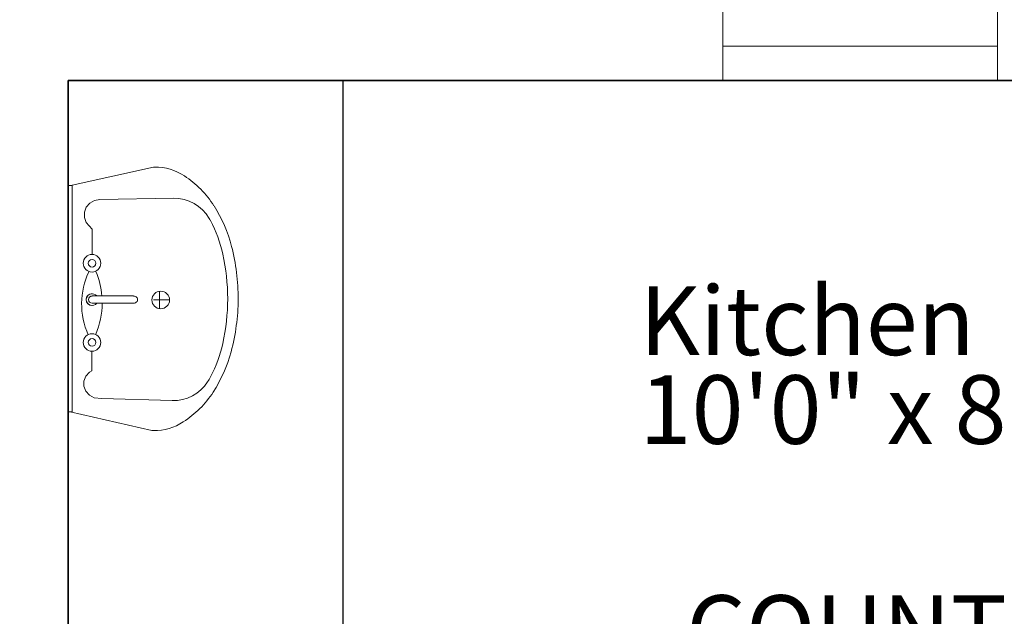
# Model space of a CAD drawing. Units: inches. Extents: x -1198 to -69, y -512 to 437.
# Tile 40 of 50: x -696 to -610, y 210 to 263. Entities that reach past the tile are written whole.
import ezdxf

# ---------------------------------------------------------------- set-up
doc = ezdxf.new("R2010")
doc.units = ezdxf.units.IN
doc.header["$MEASUREMENT"] = 0
for name, color, linetype, lineweight in [('A-ANNO-DIMS', 2, 'Continuous', 18), ('A-AREA-IDEN', 7, 'Continuous', 18), ('A-FLOR-CASE', 7, 'Continuous', 25), ('A-FLOR-FIXT', 60, 'Continuous', 18), ('A-WALL', 7, 'Continuous', 35), ('windows', 160, 'Continuous', 18)]:
    doc.layers.add(name, color=color, linetype=linetype, lineweight=lineweight)
doc.styles.get("Standard").update_dxf_attribs({"font": 'arial.ttf'})
doc.dimstyles.get("Standard").update_dxf_attribs({"dimtxt": 6, "dimasz": 6, "dimexe": 0.18, "dimexo": 0.0625, "dimgap": 0.09, "dimtad": 0, "dimtih": 1, "dimtoh": 1, "dimdec": 0, "dimzin": 0, "dimdsep": 46, "dimlunit": 4, "dimtxsty": 'Standard', "dimblk": 'OBLIQUE', "dimcen": 0.09, "dimadec": 0, "dimazin": 0, "dimtfac": 1, "dimtdec": 0, "dimtofl": 0, "dimtmove": 0, "dimatfit": 3, "dimfxl": 1, "dimtolj": 1, "dimtzin": 0, "dimarcsym": 0})

# ---------------------------------------------------------------- blocks, each defined once
blk = doc.blocks.new('A$C6AA41FE3')
at = {"linetype": 'ByBlock'}
for p, q in [((0.1919, 0.5849), (0.3733, 0.5439)), ((0.3687, 0.04), (0.3687, 0.5439)), ((0.3687, 0.5439), (0.3772, 0.5439)), ((0.3772, 0.0411), (0.3772, 0.5439)), ((0.3026, 0.514), (0.1469, 0.5187)), ((0.32, 0.5127), (0.3026, 0.514)), ((0.3305, 0.5069), (0.32, 0.5127)), ((0.3383, 0.4979), (0.3305, 0.5069)), ((0.3425, 0.4869), (0.3383, 0.4979)), ((0.3425, 0.4752), (0.3425, 0.4869)), ((0.3305, 0.4553), (0.3383, 0.4642)), ((0.3383, 0.4642), (0.3425, 0.4752)), ((0.3251, 0.409), (0.3253, 0.4524)), ((0.3253, 0.4524), (0.3305, 0.4553)), ((0.1747, 0.3146), (0.1747, 0.2774)), ((0.1525, 0.2951), (0.1884, 0.2951)), ((0.2326, 0.3025), (0.3243, 0.3025)), ((0.2326, 0.3021), (0.2326, 0.3025)), ((0.2326, 0.2863), (0.2326, 0.2867)), ((0.3243, 0.2863), (0.2326, 0.2863)), ((0.3243, 0.3025), (0.3243, 0.3024)), ((0.3243, 0.2864), (0.3243, 0.2863)), ((0.3243, 0.1379), (0.3245, 0.1941)), ((0.3374, 0.1229), (0.3243, 0.1379)), ((0.3415, 0.1119), (0.3374, 0.1229)), ((0.3415, 0.1002), (0.3415, 0.1119)), ((0.3296, 0.0802), (0.3374, 0.0892)), ((0.3374, 0.0892), (0.3415, 0.1002)), ((0.144, 0.0693), (0.3071, 0.0724)), ((0.3071, 0.0724), (0.3191, 0.0744)), ((0.3191, 0.0744), (0.3296, 0.0802)), ((0.188, 0), (0.3687, 0.04)), ((0.3772, 0.0411), (0.3687, 0.0411))]:
    blk.add_line(p, q, dxfattribs=at)
for centre, radius in [((0.3245, 0.3895), 0.0195), ((0.3245, 0.3895), 0.00849), ((0.172, 0.2951), 0.0195), ((0.3245, 0.2136), 0.0195), ((0.3245, 0.2136), 0.00849)]:
    blk.add_circle(centre, radius, dxfattribs=at)
for centre, radius, start, end in [((0.1864, 0.4671), 0.118, 89.1785, 123.1413), ((0.1877, 0.4667), 0.1183, 87.9266, 89.8113), ((0.241, 0.3799), 0.2208, 122.6461, 147.0936), ((0.1441, 0.4288), 0.09, 88.2595, 147.7588), ((0.3304, 0.324), 0.3262, 147.383, 164.6821), ((0.3272, 0.3256), 0.3003, 152.1306, 167.3001), ((0.2193, 0.3814), 0.1789, 147.7588, 151.7723), ((0.4743, 0.289), 0.4743, 165.1956, 179.4863), ((0.5, 0.2906), 0.4766, 167.7656, 179.7702), ((0.1798, 0.3042), 0.1678, 334.4875, 24.1794), ((0.4839, 0.3016), 0.1818, 157.4645, 179.7061), ((0.3243, 0.2944), 0.013, 218.4979, 141.5021), ((0.3243, 0.2944), 0.0134, 270, 90), ((0.4743, 0.2935), 0.4743, 180.0316, 194.3223), ((0.5, 0.2944), 0.4766, 180.2298, 192.2344), ((0.2312, 0.2944), 0.0078, 80.1551, 279.8449), ((0.4839, 0.3016), 0.1818, 184.8087, 202.5355), ((0.3243, 0.2944), 0.00798, 270, 90), ((0.33, 0.2597), 0.3262, 194.841, 212.14), ((0.3272, 0.2594), 0.3003, 192.6999, 207.8694), ((0.2193, 0.2037), 0.1789, 208.2281, 209.9799), ((0.1423, 0.1592), 0.09, 209.9799, 271.0537), ((0.2402, 0.2046), 0.2208, 212.4413, 236.8887), ((0.1848, 0.1179), 0.1179, 236.4084, 270.3713), ((0.1861, 0.1183), 0.1183, 269.7541, 270.9471)]:
    blk.add_arc(centre, radius, start, end, dxfattribs=at)
blk = doc.blocks.new('A1')
at = {"xscale": 1000, "yscale": 1000, "zscale": 1000, "rotation": 90}
blk.add_blockref('A$C6AA41FE3', (292.5, -377.2), dxfattribs=at)
blk = doc.blocks.new('WIN-W2-24')
at = {"ltscale": 10}
for p, q in [((0, 6), (0, 0)), ((24, 6), (24, 0)), ((0, 3), (24, 3))]:
    blk.add_line(p, q, dxfattribs=at)
blk = doc.blocks.new('COUNTER-L')
at = {"ltscale": 10}
for p, q in [((0, 96), (0, 24)), ((49.349, 24), (0, 24)), ((49.349, 0), (49.349, 24))]:
    blk.add_line(p, q, dxfattribs=at)
blk = doc.blocks.new('_Oblique')
at = {"color": 0, "linetype": 'ByBlock', "lineweight": -2}
blk.add_line((-0.5, -0.5), (0.5, 0.5), dxfattribs=at)
blk = doc.blocks.new('*D56')
at = {"layer": 'A-ANNO-DIMS', "color": 0, "lineweight": -2, "ltscale": 10, "transparency": 16777216}
for p, q in [((-618.339, 257.228), (-603.822, 257.228)), ((-604.002, 257.228), (-604.002, 212.422)), ((-604.002, 161.228), (-604.002, 206.033)), ((-618.339, 161.228), (-603.822, 161.228))]:
    blk.add_line(p, q, dxfattribs=at)
at = {"layer": 'DEFPOINTS', "color": 0, "ltscale": 10, "transparency": 16777216}
for p in [(-618.402, 257.228), (-604.002, 257.228), (-618.402, 161.228)]:
    blk.add_point(p, dxfattribs=at)
at = {"layer": 'A-ANNO-DIMS', "color": 0, "lineweight": -2, "ltscale": 10, "transparency": 16777216, "xscale": 6, "yscale": 6, "zscale": 6}
for p, rotation in [((-604.002, 257.228), 90), ((-604.002, 161.228), 270)]:
    blk.add_blockref('_Oblique', p, dxfattribs=dict(at, rotation=rotation))
at = {"layer": 'A-ANNO-DIMS', "color": 0, "ltscale": 10, "transparency": 16777216, "insert": (-604.002, 209.228), "char_height": 6, "attachment_point": 5}
blk.add_mtext('\\A1;COUNTER 96 TYP.', dxfattribs=at)
blk = doc.blocks.new('*D76')
at = {"layer": 'A-ANNO-DIMS', "color": 0, "lineweight": -2, "ltscale": 10, "transparency": 16777216}
for p, q in [((-711.132, -38.21), (-711.132, 433.184)), ((-711.132, 433.004), (-697.751, 433.004)), ((-697.751, -38.21), (-697.751, 433.184)), ((-697.751, 433.004), (-691.751, 433.004))]:
    blk.add_line(p, q, dxfattribs=at)
at = {"layer": 'DEFPOINTS', "color": 0, "ltscale": 10, "transparency": 16777216}
for p in [(-697.751, 433.004), (-711.132, -38.272), (-697.751, -38.272)]:
    blk.add_point(p, dxfattribs=at)
at = {"layer": 'A-ANNO-DIMS', "color": 0, "lineweight": -2, "ltscale": 10, "transparency": 16777216, "xscale": 6, "yscale": 6, "zscale": 6, "rotation": 180}
blk.add_blockref('_Oblique', (-711.132, 433.004), dxfattribs=at)
at = {"layer": 'A-ANNO-DIMS', "color": 0, "lineweight": -2, "ltscale": 10, "transparency": 16777216, "xscale": 6, "yscale": 6, "zscale": 6}
blk.add_blockref('_Oblique', (-697.751, 433.004), dxfattribs=at)
at = {"layer": 'A-ANNO-DIMS', "color": 0, "ltscale": 10, "transparency": 16777216, "insert": (-681.814, 433.004), "char_height": 6, "attachment_point": 5}
blk.add_mtext('\\A1;13.38', dxfattribs=at)

msp = doc.modelspace()

# ---------------------------------------------------------------- linework, layer by layer
at = {"layer": 'A-WALL', "ltscale": 10}
for p, q in [((-691.7509, 257.2277), (-691.7509, 38.2277)), ((-376.7509, 257.2277), (-691.7509, 257.2277)), ((-691.7509, 257.2277), (-691.7509, 161.2277)), ((-691.7509, 257.2277), (-601.6458, 257.2277))]:
    msp.add_line(p, q, dxfattribs=at)

# ---------------------------------------------------------------- block references
at = {"layer": 'A-FLOR-CASE'}
msp.add_blockref('COUNTER-L', (-667.751, 161.228), dxfattribs=at)
at = {"layer": 'A-FLOR-FIXT', "ltscale": 10, "xscale": 0.0393700787401575, "yscale": 0.0393700787401575, "zscale": 0.0393700787401575, "rotation": 90}
msp.add_blockref('A1', (-691.7509, 238.1491), dxfattribs=at)
at = {"layer": 'windows'}
msp.add_blockref('WIN-W2-24', (-634.559, 257.228), dxfattribs=at)

# ---------------------------------------------------------------- texts
at = {"layer": 'A-AREA-IDEN', "ltscale": 10, "char_height": 6, "attachment_point": 1}
for s, insert in [('Kitchen', (-641.8292, 239.2277)), ('10\'0" x 8\'0"', (-641.8292, 231.4637))]:
    msp.add_mtext_dynamic_manual_height_columns(s, width=57.976527, gutter_width=30, heights=[0], dxfattribs=dict(at, insert=insert))

# ---------------------------------------------------------------- dimensions: what is measured, and where the dimension line sits
at = {"layer": 'A-ANNO-DIMS', "ltscale": 10}
dim = msp.add_linear_dim(base=(-697.7509, 433.0036), p1=(-711.1319, -38.2723), p2=(-697.7509, -38.2723), dimstyle='Standard', override={"dimdec": 2, "dimlfac": 1, "dimrnd": 0, "dimzin": 0, "dimdsep": 46, "dimlunit": 2}, dxfattribs=at)
dim.commit()
dim.dimension.update_dxf_attribs({"geometry": '*D76', "text_midpoint": (-681.8137, 433.0036)})
dim = msp.add_linear_dim(base=(-604.0019, 257.2277), p1=(-618.4019, 161.2277), p2=(-618.4019, 257.2277), angle=90, text='COUNTER <> TYP.', dimstyle='Standard', override={"dimdec": 0, "dimlfac": 1, "dimrnd": 0, "dimzin": 0, "dimdsep": 46, "dimlunit": 2}, dxfattribs=at)
dim.commit()
dim.dimension.update_dxf_attribs({"geometry": '*D56', "text_midpoint": (-604.0019, 209.2277)})

doc.saveas('drawing.dxf')
